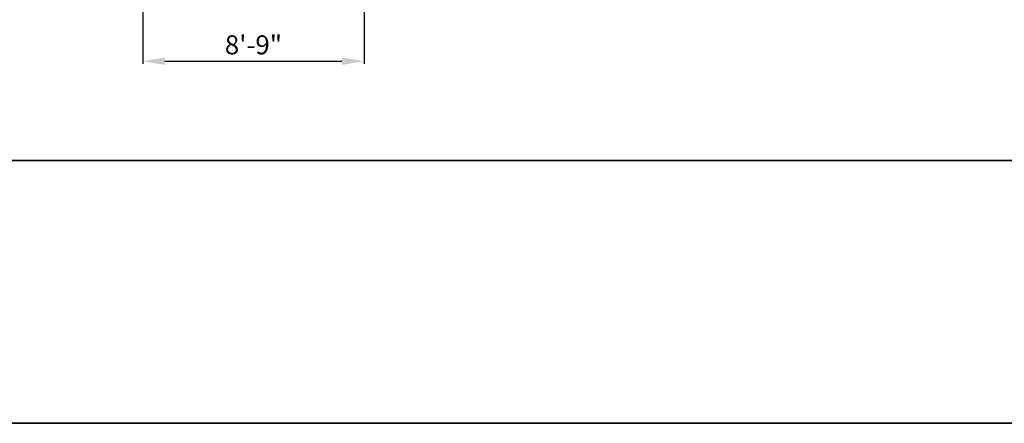
# Model space of a CAD drawing. Units: inches. Extents: x 1956 to 4770, y 1551 to 2596.
# Tile 1 of 10: x 2200 to 2667, y 1551 to 1743. Entities that reach past the tile are written whole.
import ezdxf

# ---------------------------------------------------------------- set-up
doc = ezdxf.new("R2010")
doc.units = ezdxf.units.IN
doc.layers.add('A-ANNO-DIMS', color=2, linetype='Continuous', lineweight=18)
doc.layers.add('A-ANNO-TTLB', color=7, linetype='Continuous', lineweight=35)
doc.styles.get("Standard").update_dxf_attribs({"font": 'arial.ttf'})
doc.dimstyles.new('ISO-25', dxfattribs={"dimtxt": 9, "dimasz": 10.5, "dimexe": 1.25, "dimexo": 0.625, "dimgap": 2, "dimtad": 1, "dimdec": 1, "dimlunit": 4, "dimtxsty": 'Standard', "dimcen": 2.5, "dimadec": 0, "dimazin": 0, "dimtfac": 1, "dimtdec": 1, "dimtmove": 0, "dimatfit": 3, "dimfxl": 1, "dimarcsym": 0})

# ---------------------------------------------------------------- blocks, each defined once
blk = doc.blocks.new('*D63')
at = {"layer": 'A-ANNO-DIMS', "color": 0, "lineweight": -2, "transparency": 16777216}
for p, q in [((2258.25, 1756.46), (2258.25, 1721.79)), ((2363.25, 1756.46), (2363.25, 1721.79)), ((2268.75, 1723.04), (2352.75, 1723.04))]:
    blk.add_line(p, q, dxfattribs=at)
at = {"layer": 'A-ANNO-DIMS', "color": 0, "transparency": 16777216}
for points in [[(2268.75, 1724.79), (2268.75, 1721.29), (2258.25, 1723.04)], [(2352.75, 1724.79), (2352.75, 1721.29), (2363.25, 1723.04)]]:
    blk.add_solid(points, dxfattribs=at)
at = {"layer": 'Defpoints', "color": 0, "transparency": 16777216}
for p in [(2258.25, 1757.09), (2363.25, 1757.09), (2363.25, 1723.04)]:
    blk.add_point(p, dxfattribs=at)
at = {"layer": 'A-ANNO-DIMS', "color": 0, "transparency": 16777216, "insert": (2310.75, 1729.63), "char_height": 9, "attachment_point": 5}
blk.add_mtext('8\'-9"', dxfattribs=at)

msp = doc.modelspace()

# ---------------------------------------------------------------- linework, layer by layer
at = {"layer": 'A-ANNO-TTLB'}
for points in [[(1955.79, 2596.29), (4769.89, 2596.29), (4769.89, 1551.4), (1955.79, 1551.4)], [(2042.64, 2439.33), (3293.93, 2439.33), (3293.93, 1676.04), (2042.64, 1676.04)]]:
    msp.add_lwpolyline(points, close=True, dxfattribs=at)

# ---------------------------------------------------------------- dimensions: what is measured, and where the dimension line sits
at = {"layer": 'A-ANNO-DIMS'}
dim = msp.add_linear_dim(base=(2363.25, 1723.04), p1=(2258.25, 1757.09), p2=(2363.25, 1757.09), dimstyle='ISO-25', override={"dimdec": 1, "dimlfac": 1, "dimrnd": 0, "dimzin": 1, "dimdsep": 46, "dimlunit": 4, "dimfrac": 2}, dxfattribs=at)
dim.commit()
dim.dimension.update_dxf_attribs({"geometry": '*D63', "text_midpoint": (2310.75, 1729.63)})

doc.saveas('drawing.dxf')
